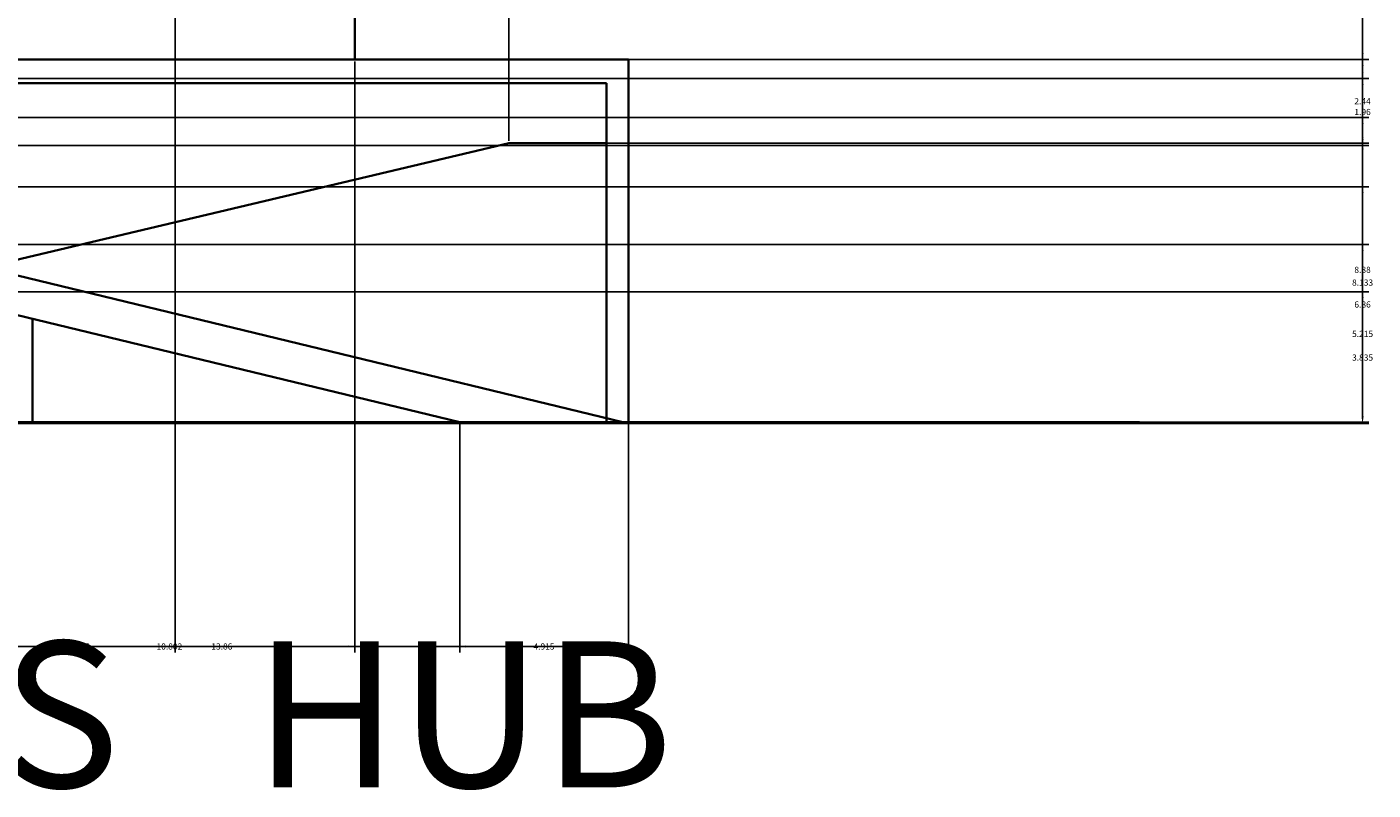
# Model space of a CAD drawing. Units: inches. Extents: x -10 to 130, y -32 to 34.
# Tile 19 of 22: x 90 to 130, y -32 to -10. Entities that reach past the tile are written whole.
import ezdxf

# ---------------------------------------------------------------- set-up
doc = ezdxf.new("R2010")
doc.units = ezdxf.units.IN
doc.header["$MEASUREMENT"] = 0
for name, color, linetype, lineweight in [('A-ANNO-DIMS', 2, 'Continuous', 18), ('A-ANNO-TEXT', 7, 'Continuous', 25), ('A-ELEV', 7, 'Continuous', 35)]:
    doc.layers.add(name, color=color, linetype=linetype, lineweight=lineweight)
doc.styles.get("Standard").update_dxf_attribs({"font": 'arial.ttf'})
doc.dimstyles.get("Standard").update_dxf_attribs({"dimtxt": 0.18, "dimasz": 0.18, "dimexe": 0.18, "dimexo": 0.0625, "dimgap": 0.09, "dimtad": 0, "dimtih": 1, "dimtoh": 1, "dimdec": 4, "dimzin": 0, "dimdsep": 46, "dimtxsty": 'Standard', "dimcen": 0.09, "dimadec": 0, "dimazin": 0, "dimtfac": 1, "dimtdec": 4, "dimtofl": 0, "dimtmove": 0, "dimatfit": 3, "dimfxl": 1, "dimtolj": 1, "dimtzin": 0, "dimarcsym": 0})

# ---------------------------------------------------------------- blocks, each defined once
blk = doc.blocks.new('*D1')
at = {"layer": 'A-ANNO-DIMS', "color": 0, "lineweight": -2, "transparency": 16777216}
for p, q in [((5.634, -13.647), (5.634, -28.129)), ((107.933, -21.477), (107.933, -28.129)), ((5.814, -27.949), (56.398, -27.949)), ((107.753, -27.949), (57.169, -27.949))]:
    blk.add_line(p, q, dxfattribs=at)
at = {"layer": 'A-ANNO-DIMS', "color": 0, "transparency": 16777216}
for points in [[(5.814, -27.919), (5.814, -27.979), (5.634, -27.949)], [(107.753, -27.919), (107.753, -27.979), (107.933, -27.949)]]:
    blk.add_solid(points, dxfattribs=at)
at = {"layer": 'Defpoints', "color": 0, "transparency": 16777216}
for p in [(5.634, -13.584), (107.933, -21.414), (107.933, -27.949)]:
    blk.add_point(p, dxfattribs=at)
at = {"layer": 'A-ANNO-DIMS', "color": 0, "transparency": 16777216, "insert": (56.784, -27.949), "char_height": 0.18, "attachment_point": 5}
blk.add_mtext('\\A1;102.3', dxfattribs=at)
blk = doc.blocks.new('*D2')
at = {"layer": 'A-ANNO-DIMS', "color": 0, "lineweight": -2, "transparency": 16777216}
for p, q in [((68.738, 27.199), (129.508, 27.199)), ((129.328, 27.019), (129.328, 3.074)), ((129.328, -21.234), (129.328, 2.71)), ((107.996, -21.414), (129.508, -21.414))]:
    blk.add_line(p, q, dxfattribs=at)
at = {"layer": 'A-ANNO-DIMS', "color": 0, "transparency": 16777216}
for points in [[(129.298, 27.019), (129.358, 27.019), (129.328, 27.199)], [(129.298, -21.234), (129.358, -21.234), (129.328, -21.414)]]:
    blk.add_solid(points, dxfattribs=at)
at = {"layer": 'Defpoints', "color": 0, "transparency": 16777216}
for p in [(68.676, 27.199), (129.328, 27.199), (107.933, -21.414)]:
    blk.add_point(p, dxfattribs=at)
at = {"layer": 'A-ANNO-DIMS', "color": 0, "transparency": 16777216, "insert": (129.328, 2.892), "char_height": 0.18, "attachment_point": 5}
blk.add_mtext('\\A1;48.61', dxfattribs=at)
blk = doc.blocks.new('*D47')
at = {"layer": 'A-ANNO-DIMS', "color": 0, "lineweight": -2, "transparency": 16777216}
for p, q in [((35.567, -12.534), (129.508, -12.534)), ((129.328, -12.714), (129.328, -16.792)), ((129.328, -21.234), (129.328, -17.156)), ((32.034, -21.414), (129.508, -21.414))]:
    blk.add_line(p, q, dxfattribs=at)
at = {"layer": 'A-ANNO-DIMS', "color": 0, "transparency": 16777216}
for points in [[(129.298, -12.714), (129.358, -12.714), (129.328, -12.534)], [(129.298, -21.234), (129.358, -21.234), (129.328, -21.414)]]:
    blk.add_solid(points, dxfattribs=at)
at = {"layer": 'Defpoints', "color": 0, "transparency": 16777216}
for p in [(35.505, -12.534), (31.971, -21.414), (129.328, -21.414)]:
    blk.add_point(p, dxfattribs=at)
at = {"layer": 'A-ANNO-DIMS', "color": 0, "transparency": 16777216, "insert": (129.328, -16.974), "char_height": 0.18, "attachment_point": 5}
blk.add_mtext('\\A1;8.88', dxfattribs=at)
blk = doc.blocks.new('*D57')
at = {"layer": 'A-ANNO-DIMS', "color": 0, "lineweight": -2, "transparency": 16777216}
for p, q in [((72.469, -14.555), (129.508, -14.555)), ((129.328, -14.735), (129.328, -17.803)), ((129.328, -21.234), (129.328, -18.167)), ((72.677, -21.414), (129.508, -21.414))]:
    blk.add_line(p, q, dxfattribs=at)
at = {"layer": 'A-ANNO-DIMS', "color": 0, "transparency": 16777216}
for points in [[(129.298, -14.735), (129.358, -14.735), (129.328, -14.555)], [(129.298, -21.234), (129.358, -21.234), (129.328, -21.414)]]:
    blk.add_solid(points, dxfattribs=at)
at = {"layer": 'Defpoints', "color": 0, "transparency": 16777216}
for p in [(72.406, -14.555), (72.614, -21.414), (129.328, -21.414)]:
    blk.add_point(p, dxfattribs=at)
at = {"layer": 'A-ANNO-DIMS', "color": 0, "transparency": 16777216, "insert": (129.328, -17.985), "char_height": 0.18, "attachment_point": 5}
blk.add_mtext('\\A1;6.86', dxfattribs=at)
blk = doc.blocks.new('*D58')
at = {"layer": 'A-ANNO-DIMS', "color": 0, "lineweight": -2, "transparency": 16777216}
for p, q in [((70.737, -16.234), (129.508, -16.234)), ((129.328, -16.414), (129.328, -18.66)), ((129.328, -21.269), (129.328, -19.024)), ((70.737, -21.449), (129.508, -21.449))]:
    blk.add_line(p, q, dxfattribs=at)
at = {"layer": 'A-ANNO-DIMS', "color": 0, "transparency": 16777216}
for points in [[(129.298, -16.414), (129.358, -16.414), (129.328, -16.234)], [(129.298, -21.269), (129.358, -21.269), (129.328, -21.449)]]:
    blk.add_solid(points, dxfattribs=at)
at = {"layer": 'Defpoints', "color": 0, "transparency": 16777216}
for p in [(70.674, -16.234), (70.674, -21.449), (129.328, -21.449)]:
    blk.add_point(p, dxfattribs=at)
at = {"layer": 'A-ANNO-DIMS', "color": 0, "transparency": 16777216, "insert": (129.328, -18.842), "char_height": 0.18, "attachment_point": 5}
blk.add_mtext('\\A1;5.215', dxfattribs=at)
blk = doc.blocks.new('*D59')
at = {"layer": 'A-ANNO-DIMS', "color": 0, "lineweight": -2, "transparency": 16777216}
for p, q in [((64.975, -17.615), (129.508, -17.615)), ((129.328, -17.795), (129.328, -19.35)), ((129.328, -21.269), (129.328, -19.714)), ((64.975, -21.449), (129.508, -21.449))]:
    blk.add_line(p, q, dxfattribs=at)
at = {"layer": 'A-ANNO-DIMS', "color": 0, "transparency": 16777216}
for points in [[(129.298, -17.795), (129.358, -17.795), (129.328, -17.615)], [(129.298, -21.269), (129.358, -21.269), (129.328, -21.449)]]:
    blk.add_solid(points, dxfattribs=at)
at = {"layer": 'Defpoints', "color": 0, "transparency": 16777216}
for p in [(64.913, -17.615), (64.913, -21.449), (129.328, -21.449)]:
    blk.add_point(p, dxfattribs=at)
at = {"layer": 'A-ANNO-DIMS', "color": 0, "transparency": 16777216, "insert": (129.328, -19.532), "char_height": 0.18, "attachment_point": 5}
blk.add_mtext('\\A1;3.835', dxfattribs=at)
blk = doc.blocks.new('*D62')
at = {"layer": 'A-ANNO-DIMS', "color": 0, "lineweight": -2, "transparency": 16777216}
for p, q in [((89.158, -21.477), (89.158, -28.129)), ((103.018, -21.477), (103.018, -28.129)), ((89.338, -27.949), (95.703, -27.949)), ((102.838, -27.949), (96.473, -27.949))]:
    blk.add_line(p, q, dxfattribs=at)
at = {"layer": 'A-ANNO-DIMS', "color": 0, "transparency": 16777216}
for points in [[(89.338, -27.919), (89.338, -27.979), (89.158, -27.949)], [(102.838, -27.919), (102.838, -27.979), (103.018, -27.949)]]:
    blk.add_solid(points, dxfattribs=at)
at = {"layer": 'Defpoints', "color": 0, "transparency": 16777216}
for p in [(89.158, -21.414), (103.018, -21.414), (103.018, -27.949)]:
    blk.add_point(p, dxfattribs=at)
at = {"layer": 'A-ANNO-DIMS', "color": 0, "transparency": 16777216, "insert": (96.088, -27.949), "char_height": 0.18, "attachment_point": 5}
blk.add_mtext('\\A1;13.86', dxfattribs=at)
blk = doc.blocks.new('*D63')
at = {"layer": 'A-ANNO-DIMS', "color": 0, "lineweight": -2, "transparency": 16777216}
for p, q in [((103.018, -21.477), (103.018, -28.129)), ((107.933, -21.477), (107.933, -28.129)), ((103.198, -27.949), (105.078, -27.949)), ((107.753, -27.949), (105.874, -27.949))]:
    blk.add_line(p, q, dxfattribs=at)
at = {"layer": 'A-ANNO-DIMS', "color": 0, "transparency": 16777216}
for points in [[(103.198, -27.919), (103.198, -27.979), (103.018, -27.949)], [(107.753, -27.919), (107.753, -27.979), (107.933, -27.949)]]:
    blk.add_solid(points, dxfattribs=at)
at = {"layer": 'Defpoints', "color": 0, "transparency": 16777216}
for p in [(103.018, -21.414), (107.933, -21.414), (107.933, -27.949)]:
    blk.add_point(p, dxfattribs=at)
at = {"layer": 'A-ANNO-DIMS', "color": 0, "transparency": 16777216, "insert": (105.476, -27.949), "char_height": 0.18, "attachment_point": 5}
blk.add_mtext('\\A1;4.915', dxfattribs=at)
blk = doc.blocks.new('*D66')
at = {"layer": 'A-ANNO-DIMS', "color": 0, "lineweight": -2, "transparency": 16777216}
for p, q in [((89.158, -16.844), (89.158, 33.879)), ((104.453, -13.219), (104.453, 33.879)), ((89.338, 33.699), (96.35, 33.699)), ((104.273, 33.699), (97.261, 33.699))]:
    blk.add_line(p, q, dxfattribs=at)
at = {"layer": 'A-ANNO-DIMS', "color": 0, "transparency": 16777216}
for points in [[(89.338, 33.729), (89.338, 33.669), (89.158, 33.699)], [(104.273, 33.729), (104.273, 33.669), (104.453, 33.699)]]:
    blk.add_solid(points, dxfattribs=at)
at = {"layer": 'Defpoints', "color": 0, "transparency": 16777216}
for p in [(104.453, 33.699), (104.453, -13.282), (89.158, -16.906)]:
    blk.add_point(p, dxfattribs=at)
at = {"layer": 'A-ANNO-DIMS', "color": 0, "transparency": 16777216, "insert": (96.805, 33.699), "char_height": 0.18, "attachment_point": 5}
blk.add_mtext('\\A1;15.295', dxfattribs=at)
blk = doc.blocks.new('*D67')
at = {"layer": 'A-ANNO-DIMS', "color": 0, "lineweight": -2, "transparency": 16777216}
for p, q in [((104.516, -13.282), (129.508, -13.282)), ((129.328, -13.462), (129.328, -17.166)), ((129.328, -21.234), (129.328, -17.53)), ((107.996, -21.414), (129.508, -21.414))]:
    blk.add_line(p, q, dxfattribs=at)
at = {"layer": 'A-ANNO-DIMS', "color": 0, "transparency": 16777216}
for points in [[(129.298, -13.462), (129.358, -13.462), (129.328, -13.282)], [(129.298, -21.234), (129.358, -21.234), (129.328, -21.414)]]:
    blk.add_solid(points, dxfattribs=at)
at = {"layer": 'Defpoints', "color": 0, "transparency": 16777216}
for p in [(104.453, -13.282), (107.933, -21.414), (129.328, -21.414)]:
    blk.add_point(p, dxfattribs=at)
at = {"layer": 'A-ANNO-DIMS', "color": 0, "transparency": 16777216, "insert": (129.328, -17.348), "char_height": 0.18, "attachment_point": 5}
blk.add_mtext('\\A1;8.133', dxfattribs=at)
blk = doc.blocks.new('*D68')
at = {"layer": 'A-ANNO-DIMS', "color": 0, "lineweight": -2, "transparency": 16777216}
for p, q in [((107.996, -10.843), (129.508, -10.843)), ((129.328, -11.023), (129.328, -11.882)), ((129.328, -13.102), (129.328, -12.243)), ((107.362, -13.282), (129.508, -13.282))]:
    blk.add_line(p, q, dxfattribs=at)
at = {"layer": 'A-ANNO-DIMS', "color": 0, "transparency": 16777216}
for points in [[(129.298, -11.023), (129.358, -11.023), (129.328, -10.843)], [(129.298, -13.102), (129.358, -13.102), (129.328, -13.282)]]:
    blk.add_solid(points, dxfattribs=at)
at = {"layer": 'Defpoints', "color": 0, "transparency": 16777216}
for p in [(107.933, -10.843), (107.3, -13.282), (129.328, -13.282)]:
    blk.add_point(p, dxfattribs=at)
at = {"layer": 'A-ANNO-DIMS', "color": 0, "transparency": 16777216, "insert": (129.328, -12.063), "char_height": 0.18, "attachment_point": 5}
blk.add_mtext('\\A1;2.44', dxfattribs=at)
blk = doc.blocks.new('*D75')
at = {"layer": 'A-ANNO-DIMS', "color": 0, "lineweight": -2, "transparency": 16777216}
for p, q in [((62.588, -11.398), (129.508, -11.398)), ((129.328, -11.578), (129.328, -12.195)), ((129.328, -13.176), (129.328, -12.559)), ((62.588, -13.356), (129.508, -13.356))]:
    blk.add_line(p, q, dxfattribs=at)
at = {"layer": 'A-ANNO-DIMS', "color": 0, "transparency": 16777216}
for points in [[(129.298, -11.578), (129.358, -11.578), (129.328, -11.398)], [(129.298, -13.176), (129.358, -13.176), (129.328, -13.356)]]:
    blk.add_solid(points, dxfattribs=at)
at = {"layer": 'Defpoints', "color": 0, "transparency": 16777216}
for p in [(62.526, -11.398), (129.328, -11.398), (62.526, -13.356)]:
    blk.add_point(p, dxfattribs=at)
at = {"layer": 'A-ANNO-DIMS', "color": 0, "transparency": 16777216, "insert": (129.328, -12.377), "char_height": 0.18, "attachment_point": 5}
blk.add_mtext('\\A1;1.96', dxfattribs=at)
blk = doc.blocks.new('*D76')
at = {"layer": 'A-ANNO-DIMS', "color": 0, "lineweight": -2, "transparency": 16777216}
for p, q in [((62.588, -6.485), (129.508, -6.485)), ((129.328, -6.665), (129.328, -8.76)), ((129.328, -11.218), (129.328, -9.123)), ((62.588, -11.398), (129.508, -11.398))]:
    blk.add_line(p, q, dxfattribs=at)
at = {"layer": 'A-ANNO-DIMS', "color": 0, "transparency": 16777216}
for points in [[(129.298, -6.665), (129.358, -6.665), (129.328, -6.485)], [(129.298, -11.218), (129.358, -11.218), (129.328, -11.398)]]:
    blk.add_solid(points, dxfattribs=at)
at = {"layer": 'Defpoints', "color": 0, "transparency": 16777216}
for p in [(62.526, -6.485), (129.328, -6.485), (62.526, -11.398)]:
    blk.add_point(p, dxfattribs=at)
at = {"layer": 'A-ANNO-DIMS', "color": 0, "transparency": 16777216, "insert": (129.328, -8.942), "char_height": 0.18, "attachment_point": 5}
blk.add_mtext('\\A1;4.913', dxfattribs=at)
blk = doc.blocks.new('*D159')
at = {"layer": 'A-ANNO-DIMS', "color": 0, "lineweight": -2, "transparency": 16777216}
for p, q in [((89.158, -6.284), (89.158, -28.129)), ((94.73, -6.284), (94.73, -28.129)), ((89.338, -27.949), (91.551, -27.949)), ((94.55, -27.949), (92.337, -27.949))]:
    blk.add_line(p, q, dxfattribs=at)
at = {"layer": 'A-ANNO-DIMS', "color": 0, "transparency": 16777216}
for points in [[(89.338, -27.919), (89.338, -27.979), (89.158, -27.949)], [(94.55, -27.919), (94.55, -27.979), (94.73, -27.949)]]:
    blk.add_solid(points, dxfattribs=at)
at = {"layer": 'Defpoints', "color": 0, "transparency": 16777216}
for p in [(89.158, -6.222), (94.73, -6.222), (94.73, -27.949)]:
    blk.add_point(p, dxfattribs=at)
at = {"layer": 'A-ANNO-DIMS', "color": 0, "transparency": 16777216, "insert": (91.944, -27.949), "char_height": 0.18, "attachment_point": 5}
blk.add_mtext('\\A1;5.572', dxfattribs=at)
blk = doc.blocks.new('*D173')
at = {"layer": 'A-ANNO-DIMS', "color": 0, "lineweight": -2, "transparency": 16777216}
for p, q in [((89.158, -10.906), (89.158, -28.129)), ((99.96, -10.906), (99.96, -28.129)), ((89.338, -27.949), (94.105, -27.949)), ((99.78, -27.949), (95.013, -27.949))]:
    blk.add_line(p, q, dxfattribs=at)
at = {"layer": 'A-ANNO-DIMS', "color": 0, "transparency": 16777216}
for points in [[(89.338, -27.919), (89.338, -27.979), (89.158, -27.949)], [(99.78, -27.919), (99.78, -27.979), (99.96, -27.949)]]:
    blk.add_solid(points, dxfattribs=at)
at = {"layer": 'Defpoints', "color": 0, "transparency": 16777216}
for p in [(89.158, -10.843), (99.96, -10.843), (99.96, -27.949)]:
    blk.add_point(p, dxfattribs=at)
at = {"layer": 'A-ANNO-DIMS', "color": 0, "transparency": 16777216, "insert": (94.559, -27.949), "char_height": 0.18, "attachment_point": 5}
blk.add_mtext('\\A1;10.802', dxfattribs=at)
blk = doc.blocks.new('*D174')
at = {"layer": 'A-ANNO-DIMS', "color": 0, "lineweight": -2, "transparency": 16777216}
for p, q in [((100.023, -6.222), (129.508, -6.222)), ((129.328, -6.402), (129.328, -8.351)), ((129.328, -10.663), (129.328, -8.715)), ((100.023, -10.843), (129.508, -10.843))]:
    blk.add_line(p, q, dxfattribs=at)
at = {"layer": 'A-ANNO-DIMS', "color": 0, "transparency": 16777216}
for points in [[(129.298, -6.402), (129.358, -6.402), (129.328, -6.222)], [(129.298, -10.663), (129.358, -10.663), (129.328, -10.843)]]:
    blk.add_solid(points, dxfattribs=at)
at = {"layer": 'Defpoints', "color": 0, "transparency": 16777216}
for p in [(99.96, -6.222), (99.96, -10.843), (129.328, -10.843)]:
    blk.add_point(p, dxfattribs=at)
at = {"layer": 'A-ANNO-DIMS', "color": 0, "transparency": 16777216, "insert": (129.328, -8.533), "char_height": 0.18, "attachment_point": 5}
blk.add_mtext('\\A1;4.622', dxfattribs=at)

msp = doc.modelspace()

# ---------------------------------------------------------------- linework, layer by layer
at = {"layer": 'A-ELEV'}
for p, q in [((99.9603, -6.2218), (99.9603, -10.8435)), ((89.1578, -10.8435), (107.9333, -10.8435)), ((107.9333, -10.8435), (107.9333, -21.4145)), ((89.1578, -11.5395), (107.2998, -11.5395)), ((107.2998, -11.5395), (107.2998, -21.4145)), ((104.4531, -13.2819), (89.1578, -16.9063)), ((107.2998, -13.2819), (104.4531, -13.2819)), ((82.377, -15.2645), (107.7767, -21.4145)), ((82.377, -16.4166), (103.0183, -21.4145)), ((90.5739, -18.4013), (90.5739, -21.4145)), ((89.1578, -21.4145), (99.9603, -21.4145)), ((99.9603, -21.4145), (122.8277, -21.4145))]:
    msp.add_line(p, q, dxfattribs=at)

# ---------------------------------------------------------------- texts
at = {"layer": 'A-ANNO-TEXT'}
msp.add_text('REAR   ELEVATION    AND   LOGISTICS   HUB', height=4.256275, dxfattribs=at).set_placement((-5.4651, -32.0569))

# ---------------------------------------------------------------- dimensions: what is measured, and where the dimension line sits
at = {"layer": 'A-ANNO-DIMS'}
for base, p1, p2, override, picture, middle in [((104.4531, 33.6987), (89.1578, -16.9063), (104.4531, -13.2819), {"dimdec": 3, "dimlfac": 1, "dimrnd": 0, "dimzin": 0, "dimdsep": 46, "dimlunit": 2}, '*D66', (96.8055, 33.6987)), ((94.7302, -27.9493), (89.1578, -6.2218), (94.7302, -6.2218), {"dimdec": 3, "dimlfac": 1, "dimrnd": 0, "dimzin": 0, "dimdsep": 46, "dimlunit": 2}, '*D159', (91.944, -27.9493)), ((99.96027, -27.9493), (89.15784, -10.84347), (99.96027, -10.84347), {"dimdec": 3, "dimlfac": 1, "dimrnd": 0, "dimzin": 0, "dimdsep": 46, "dimlunit": 2}, '*D173', (94.55905, -27.9493)), ((107.9333, -27.9493), (5.634, -13.5841), (107.9333, -21.4145), {"dimdec": 1, "dimlfac": 1, "dimrnd": 0, "dimzin": 0, "dimdsep": 46, "dimlunit": 2}, '*D1', (56.7837, -27.9493)), ((103.0183, -27.9493), (89.1578, -21.4145), (103.0183, -21.4145), {"dimdec": 2, "dimlfac": 1, "dimrnd": 0, "dimzin": 0, "dimdsep": 46, "dimlunit": 2}, '*D62', (96.0881, -27.9493)), ((107.9333, -27.9493), (103.0183, -21.4145), (107.9333, -21.4145), {"dimdec": 3, "dimlfac": 1, "dimrnd": 0, "dimzin": 0, "dimdsep": 46, "dimlunit": 2}, '*D63', (105.4758, -27.9493))]:
    dim = msp.add_linear_dim(base=base, p1=p1, p2=p2, dimstyle='Standard', override=override, dxfattribs=at)
    dim.commit()
    dim.dimension.update_dxf_attribs({"geometry": picture, "text_midpoint": middle})
for base, p1, p2, override, picture, middle in [((129.3277, 27.1987), (107.9333, -21.4145), (68.6759, 27.1987), {"dimdec": 2, "dimlfac": 1, "dimrnd": 0, "dimzin": 0, "dimdsep": 46, "dimlunit": 2}, '*D2', (129.3277, 2.8921)), ((129.3277, -10.8435), (99.9603, -6.2218), (99.9603, -10.8435), {"dimdec": 3, "dimlfac": 1, "dimrnd": 0, "dimzin": 0, "dimdsep": 46, "dimlunit": 2}, '*D174', (129.3277, -8.5326)), ((129.3277, -6.4849), (62.5256, -11.3982), (62.5256, -6.4849), {"dimdec": 3, "dimlfac": 1, "dimrnd": 0, "dimzin": 0, "dimdsep": 46, "dimlunit": 2}, '*D76', (129.3277, -8.9415)), ((129.3277, -13.2819), (107.9333, -10.8435), (107.2998, -13.2819), {"dimdec": 2, "dimlfac": 1, "dimrnd": 0, "dimzin": 0, "dimdsep": 46, "dimlunit": 2}, '*D68', (129.3277, -12.0627)), ((129.3277, -11.3982), (62.5256, -13.3558), (62.5256, -11.3982), {"dimdec": 2, "dimlfac": 1, "dimrnd": 0, "dimzin": 0, "dimdsep": 46, "dimlunit": 2}, '*D75', (129.3277, -12.377)), ((129.3277, -21.4145), (35.5046, -12.5339), (31.9712, -21.4145), {"dimdec": 2, "dimlfac": 1, "dimrnd": 0, "dimzin": 0, "dimdsep": 46, "dimlunit": 2}, '*D47', (129.3277, -16.9742)), ((129.3277, -21.4145), (104.4531, -13.2819), (107.9333, -21.4145), {"dimdec": 3, "dimlfac": 1, "dimrnd": 0, "dimzin": 0, "dimdsep": 46, "dimlunit": 2}, '*D67', (129.3277, -17.3482)), ((129.3277, -21.4145), (72.4063, -14.555), (72.6144, -21.4145), {"dimdec": 2, "dimlfac": 1, "dimrnd": 0, "dimzin": 0, "dimdsep": 46, "dimlunit": 2}, '*D57', (129.3277, -17.9847)), ((129.3277, -21.4493), (70.6743, -16.2341), (70.6743, -21.4493), {"dimdec": 3, "dimlfac": 1, "dimrnd": 0, "dimzin": 0, "dimdsep": 46, "dimlunit": 2}, '*D58', (129.3277, -18.8417)), ((129.3277, -21.4493), (64.913, -17.6146), (64.913, -21.4493), {"dimdec": 3, "dimlfac": 1, "dimrnd": 0, "dimzin": 0, "dimdsep": 46, "dimlunit": 2}, '*D59', (129.3277, -19.532))]:
    dim = msp.add_linear_dim(base=base, p1=p1, p2=p2, angle=90, dimstyle='Standard', override=override, dxfattribs=at)
    dim.commit()
    dim.dimension.update_dxf_attribs({"geometry": picture, "text_midpoint": middle})

doc.saveas('drawing.dxf')
